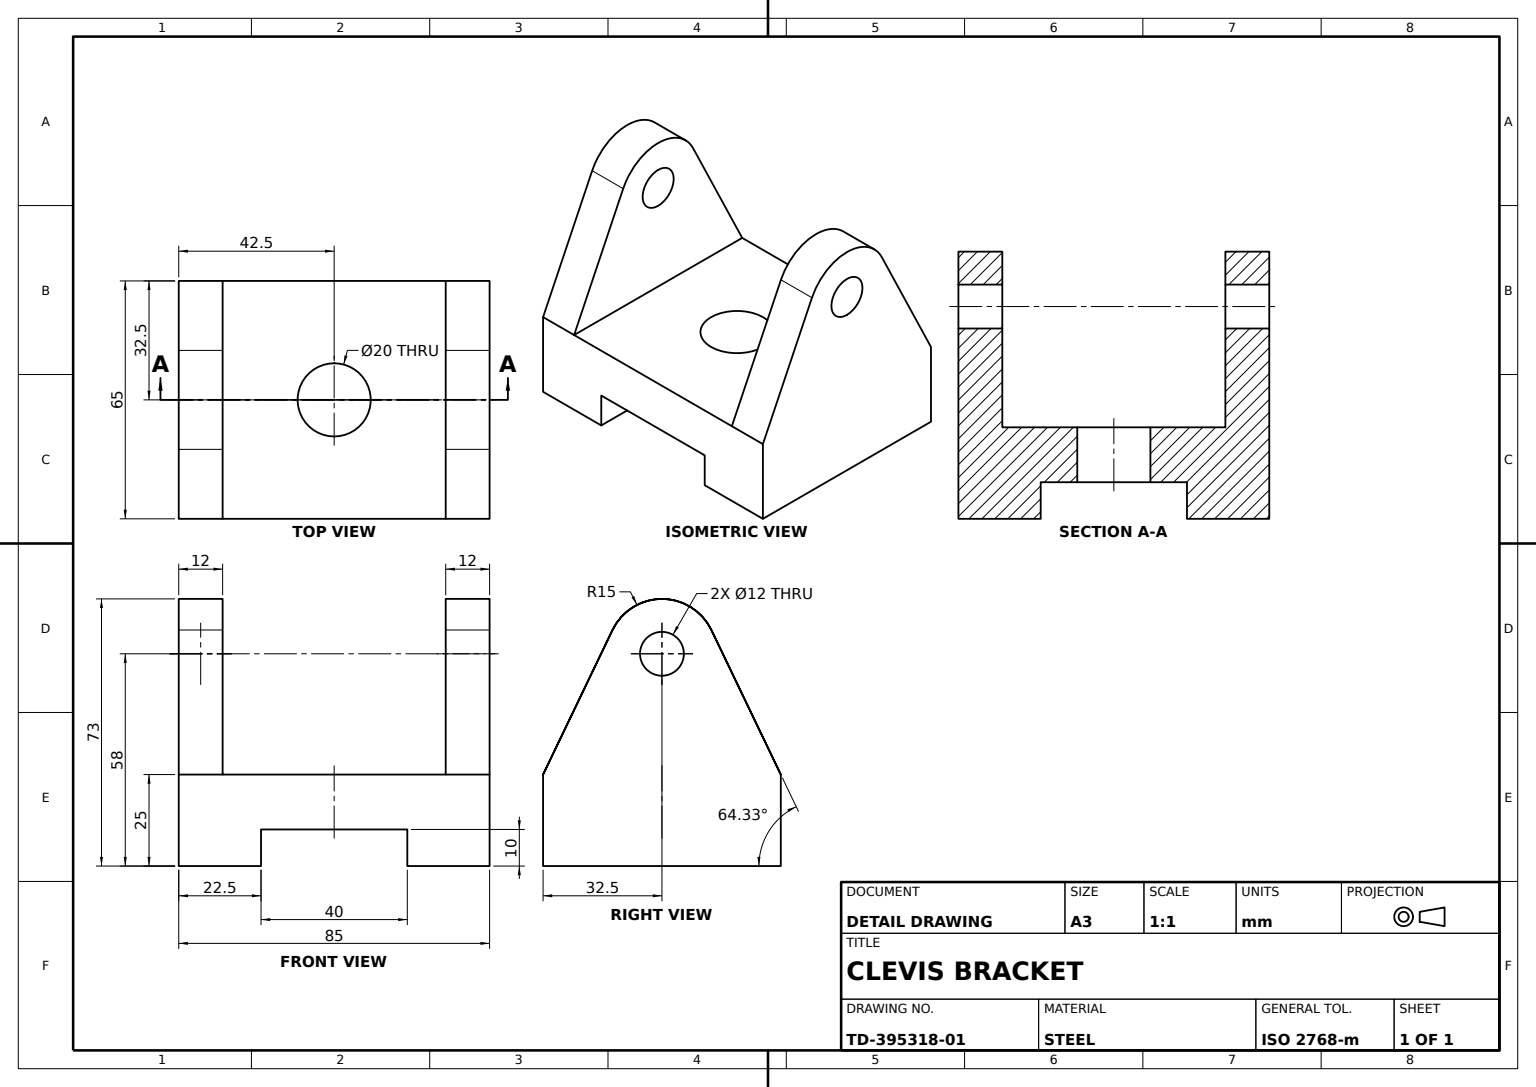
SolidWorks part; units mm, degrees
material "Plain Carbon Steel"
ref_plane "Front Plane" through (0, 0, 0) normal (0, 0, 1) x (1, 0, 0)
ref_plane "Top Plane" through (0, 0, 0) normal (0, 1, 0) x (1, 0, 0)
ref_plane "Right Plane" through (0, 0, 0) normal (1, 0, 0) x (0, 0, -1)
sketch "Base Profile Sketch" plane through (0, 0, 0) normal (0, 0, 1) x (1, 0, 0)
  line L0 (42.5, -29) -> (42.5, -4) construction
  line L1 (-42.5, 29) -> (-30.5, 29)
  line L2 (-42.5, 29) -> (-42.5, -29)
  line L3 (-42.5, -29) -> (-20, -29)
  line L4 (42.5, 29) -> (42.5, -29)
  line L5 (-42.5, 29) -> (42.5, -29) construction
  line L6 (-42.5, -29) -> (42.5, 29) construction
  line L7 (30.5, -4) -> (-30.5, -4)
  line L8 (42.5, 29) -> (30.5, 29) construction
  line L9 (20, -29) -> (20, -19)
  line L10 (20, -19) -> (-20, -19)
  line L11 (-20, -19) -> (-20, -29)
  line L12 (20, -29) -> (42.5, -29)
  line L13 (30.5, 29) -> (30.5, -4)
  line L14 (0, 0) -> (0, 29) construction
  line L15 (-30.5, 29) -> (-30.5, -4)
  line L16 (30.5, 29) -> (42.5, 29)
  point P0 (0, 0)
  dimension "D1" = 85
  dimension "D2" = 58
  dimension "D3" = 40
  dimension "D4" = 10
  dimension "D5" = 25
  dimension "D6" = 20
  dimension "D7" = 12
extrude "Base Block" add sketch "Base Profile Sketch" along normal mid plane 65
sketch "Centre Hole Sketch" plane through (0, -4, 0) normal (0, 1, 0) x (1, 0, 0)
  circle A0 centre (0, 0) radius 10
  dimension "D1" = 20
extrude "Centre Hole Ø20" cut sketch "Centre Hole Sketch" against normal blind 65
sketch "Lug A Sketch" plane through (42.5, 0, 0) normal (1, 0, 0) x (0, 0, -1)
  line L0 (-32.5, 29) -> (32.5, 29) construction
  line L1 (-32.5, -29) -> (-32.5, -4) construction
  line L2 (-32.5, -4) -> (-13.52, 35.4969)
  line L3 (0, 0) -> (0, 29) construction
  line L4 (32.5, -4) -> (13.52, 35.4969)
  line L5 (-32.5, -4) -> (32.5, -4)
  circle A0 centre (0, 29) radius 6
  circle A1 centre (0, 29) radius 15
  line M4 (32.5, 29) -> (-32.5, 29)
  dimension "D1" = 12
  dimension "D2" = 30
extrude "Lug A Boss" add sketch "Lug A Sketch" against normal blind 12 contours A1 A0 M4 | A1 A0 M4 | A1 L2 L5 L4 M4 | A1 L2 M4 | A1 L4 M4
sketch "Lug Trim Sketch" plane through (42.5, 0, 0) normal (1, 0, 0) x (0, 0, -1)
  line L0 (-32.5, -29) -> (-32.5, -17) construction
  line L1 (-32.5, -29) -> (-32.5, 29) construction
  line L2 (-32.5, -17) -> (-16.642, 29)
  line L3 (-32.5, -17) -> (-32.5, 29)
  line L4 (-32.5, 29) -> (-16.642, 29)
  line L5 (0, 0) -> (0, 29) construction
  line L6 (-6, 29) -> (6, 29) construction
  line L7 (32.5, -17) -> (16.642, 29)
  line L8 (32.5, -17) -> (32.5, 29)
  line L9 (32.5, 29) -> (16.642, 29)
  line L11 (16.642, 29) -> (32.5, 29) construction
  dimension "D1" = 46
extrude "Lug Trim Cut" cut sketch "Lug Trim Sketch" against normal through all
sketch "Lug B Sketch" plane through (42.5, 0, 0) normal (1, 0, 0) x (0, 0, -1)
  line L0 (-32.5, -29) -> (-32.5, -4) construction
  line L1 (-32.5, -4) -> (-16.642, 29) construction
  line L2 (-16.642, 29) -> (-32.5, -17) construction
  line L3 (0, 0) -> (0, 35) construction
  line L4 (-16.642, 29) -> (-32.5, -4)
  line L5 (-32.5, -4) -> (-32.5, -17)
  line L6 (-32.5, -17) -> (-16.642, 29)
  line L7 (32.5, -4) -> (32.5, -17)
  line L8 (16.642, 29) -> (32.5, -4)
  line L9 (32.5, -17) -> (16.642, 29)
  line L10 (-32.5, -29) -> (32.5, -29) construction
  arc A0 (6, 29) -> (-6, 29) centre (0, 29) ccw construction
  dimension "D1" = 25
extrude "Lug B Boss" add sketch "Lug B Sketch" against normal blind 12
sketch "Pin Hole Sketch" plane through (42.5, 0, 0) normal (1, 0, 0) x (0, 0, -1)
  line L0 (-6, 29) -> (6, 29) construction
  circle A0 centre (0, 29) radius 6
  dimension "D1" = 12
extrude "Pin Hole Cut" cut sketch "Pin Hole Sketch" against normal through all
sketch "Lug C Sketch" plane through (-42.5, 0, 0) normal (-1, 0, 0) x (0, 0, 1)
  line L0 (-32.5, -17) -> (-32.5, -4)
  line L2 (32.5, -17) -> (32.5, -4)
  line L4 (-32.5, -4) -> (-16.642, 29)
  line L5 (-16.642, 29) -> (-32.5, -17)
  line L6 (-16.642, 29) -> (-13.52, 35.4969)
  line L7 (-16.642, 29) -> (-15, 29)
  line L8 (-15, 29) -> (-6, 29)
  line L10 (32.5, -4) -> (16.642, 29)
  line L11 (16.642, 29) -> (32.5, -17)
  line L12 (15, 29) -> (6, 29)
  line L13 (16.642, 29) -> (13.52, 35.4969)
  line L14 (-15, 29) -> (-16.642, 29)
  line L15 (15, 29) -> (16.642, 29)
  arc A0 (-13.52, 35.4969) -> (-15, 29) centre (0, 29) ccw
  circle A1 centre (0, 29) radius 6
  arc A3 (13.52, 35.4969) -> (15, 29) centre (0, 29) cw
  arc A4 (15, 29) -> (-15, 29) centre (0, 29) ccw
  line M7 (16.642, 29) -> (6, 29)
  line M9 (-6, 29) -> (-16.642, 29)
  line M10 (-16.642, 29) -> (-32.5, -17)
  line M14 (32.5, -17) -> (16.642, 29)
extrude "Lug C Boss" add sketch "Lug C Sketch" against normal blind 12 contours A3 A4 A0 A1 M9 M7 | L4 L0 M10 | L2 L10 M14 | A0 L6 M9 | L13 A3 M7
sketch "Lug Rib A Sketch" plane through (0, -4, 0) normal (0, 1, 0) x (1, 0, 0)
  line L0 (-30.5, 32.5) -> (30.5, 32.5)
  line L1 (30.5, 32.5) -> (30.5, 28.0184)
  line L2 (30.5, 28.0184) -> (-30.5, 28.0184)
  line L3 (-30.5, 28.0184) -> (-30.5, 32.5)
extrude "Lug Rib A" add sketch "Lug Rib A Sketch" against normal blind 13
sketch "Lug Rib B Sketch" plane through (0, -4, 0) normal (0, 1, 0) x (1, 0, 0)
  line L0 (-30.5, -28.0184) -> (-30.5, -32.5)
  line L1 (-30.5, -32.5) -> (30.5, -32.5)
  line L2 (30.5, -32.5) -> (30.5, -28.0184)
  line L3 (30.5, -28.0184) -> (-30.5, -28.0184)
extrude "Lug Rib B" add sketch "Lug Rib B Sketch" against normal blind 13
